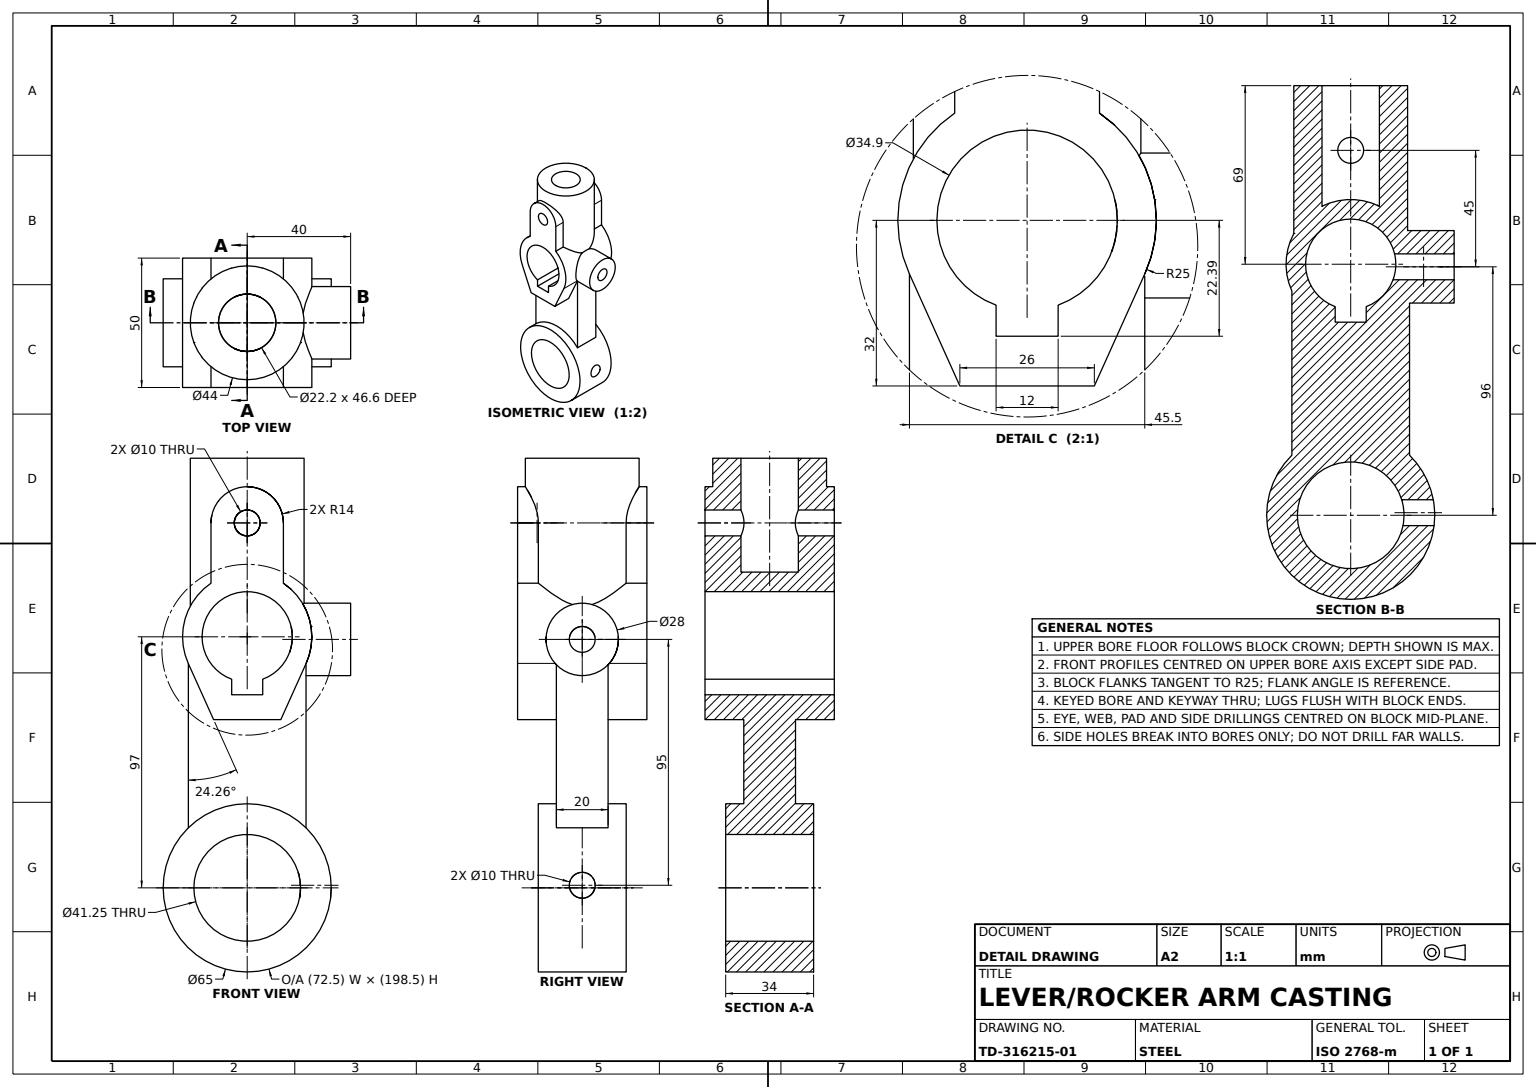
from build123d import *

# Parameters (mm, degrees)
CENTER_BLOCK_DEPTH             = 25
LOWER_EYE_PROFILE_65_R         = 32.5
LOWER_EYE_BOSS_65_DEPTH        = 17
CONNECTING_ARM_PROFILE_W       = 20
CONNECTING_ARM_PROFILE_H       = 65
CONNECTING_ARM_DEPTH           = 22.75
UPPER_BOSS_44_REACH            = 204.691
UPPER_BOSS_44_END_RADIUS       = 25
UPPER_BOSS_PROFILE_44_R        = 22
SIDE_PAD_REACH                 = 144.571
SIDE_PAD_END_RADIUS            = 22
SIDE_PAD_EXTENSION_REACH       = 144.571
UPPER_BORE_22_2_REACH          = 204.691
UPPER_BORE_22_2_END_RADIUS     = 25
UPPER_BORE_PROFILE_22_2_R      = 11.1
LUG_PLATE_REACH                = 152.504
LUG_PLATE_PROFILE_R            = 14
KEYED_SIDE_BORE_PROFILE_R      = 5
KEYED_SIDE_BORE_DEPTH          = 145.465393842
LUG_PIN_HOLE_PROFILE_10_R      = 5
LUG_PIN_HOLE_10_DEPTH          = 45
LOWER_EYE_BORE_PROFILE_41_25_R = 20.625
LOWER_EYE_BORE_41_25_DEPTH     = 45
CROSS_PIN_HOLE_PROFILE_10_R    = 5
CROSS_PIN_HOLE_10_DEPTH        = 100


with BuildPart() as part:
    # Center Block Profile → Center Block (new, symmetric)
    with BuildSketch(Plane.XY):
        with BuildLine():
            Line((-13, -32), (13, -32))
            Line((13, -32), (22.792288735, -10.271882702))
            ThreePointArc((22.792288735, -10.271882702), (0, 25), (-22.792288735, -10.271882702))
            Line((-22.792288735, -10.271882702), (-13, -32))
        make_face()
    extrude(amount=CENTER_BLOCK_DEPTH, both=True)



with BuildPart() as body_2:
    # Lower Eye Profile Ø65 → Lower Eye Boss Ø65 (new, symmetric)
    with BuildSketch(Plane.XY):
        with Locations((0, -97)):
            Circle(LOWER_EYE_PROFILE_65_R)
    extrude(amount=LOWER_EYE_BOSS_65_DEPTH, both=True)


with BuildPart() as part_1:
    add(part.part)

    add(body_2.part)  # Connecting Arm merges body 2
    # Connecting Arm Profile → Connecting Arm (add, symmetric)
    with BuildSketch(Plane(origin=(0, 0, 0), x_dir=(0, 0, -1), z_dir=(1, 0, 0))):
        with Locations((0, -42.771882702)):
            Rectangle(CONNECTING_ARM_PROFILE_W, CONNECTING_ARM_PROFILE_H)
    extrude(amount=CONNECTING_ARM_DEPTH, both=True)

    # Upper Boss Ø44: up to this cylinder (the profile starts outside it)
    upper_boss_44_end = Plane(origin=(0, 0, 0), z_dir=(0, 0, -1)) * Cylinder(UPPER_BOSS_44_END_RADIUS, 460.382, mode=Mode.PRIVATE)
    # Upper Boss Profile Ø44 → Upper Boss Ø44 (add, up to the surface)
    with BuildSketch(Plane(origin=(0, 69, 0), x_dir=(1, 0, 0), z_dir=(0, 1, 0)), mode=Mode.PRIVATE) as upper_boss_44_sk1:
        with Locations(Location((0, 0, 0), (0, 0, 270))):
            Circle(UPPER_BOSS_PROFILE_44_R)
    upper_boss_44_tool1 = extrude(upper_boss_44_sk1.sketch, amount=-UPPER_BOSS_44_REACH, mode=Mode.PRIVATE) - upper_boss_44_end
    add(upper_boss_44_tool1.solids().sort_by_distance((0, 69, 0))[0])

    # Side Pad: up to this cylinder (the profile starts outside it)
    side_pad_end = Plane(origin=(0, 39.439951, 0), z_dir=(0, 1, 0)) * Cylinder(SIDE_PAD_END_RADIUS, 334.142, mode=Mode.PRIVATE)
    # Side Pad Profile → Side Pad (add, up to the surface)
    with BuildSketch(Plane.XY.offset(25), mode=Mode.PRIVATE) as side_pad_sk1:
        with BuildLine():
            Line((-14, 44), (-14, 20.712315177))
            ThreePointArc((-14, 20.712315177), (0, 25), (14, 20.712315177))
            Line((14, 20.712315177), (14, 44))
            ThreePointArc((14, 44), (0, 58), (-14, 44))
        make_face()
    side_pad_tool1 = extrude(side_pad_sk1.sketch, amount=-SIDE_PAD_REACH, mode=Mode.PRIVATE) - side_pad_end
    add(side_pad_tool1.solids().sort_by_distance((0, 39.439951, 25))[0])

    # Side Pad Extension Profile → Side Pad Extension (add, up to next)
    with BuildSketch(Plane(origin=(0, 0, -25), x_dir=(-1, 0, 0), z_dir=(0, 0, -1)), mode=Mode.PRIVATE) as side_pad_extension_sk1:
        with BuildLine():
            Line((-14, 44), (-14, 20.712315177))
            ThreePointArc((-14, 20.712315177), (0, 25), (14, 20.712315177))
            Line((14, 20.712315177), (14, 44))
            ThreePointArc((14, 44), (0, 58), (-14, 44))
        make_face()
    side_pad_extension_tool1 = extrude(side_pad_extension_sk1.sketch, amount=-SIDE_PAD_EXTENSION_REACH, mode=Mode.PRIVATE) - part_1.part
    add(side_pad_extension_tool1.solids().sort_by_distance((0, 39.439951, -25))[0])

    # Upper Bore Ø22.2: up to this cylinder (the profile starts outside it)
    upper_bore_22_2_end = Plane(origin=(0, 0, 0), z_dir=(0, 0, -1)) * Cylinder(UPPER_BORE_22_2_END_RADIUS, 460.382, mode=Mode.PRIVATE)
    # Upper Bore Profile Ø22.2 → Upper Bore Ø22.2 (cut, up to the surface)
    with BuildSketch(Plane(origin=(0, 69, 0), x_dir=(1, 0, 0), z_dir=(0, 1, 0)), mode=Mode.PRIVATE) as upper_bore_22_2_sk1:
        with Locations(Location((0, 0, 0), (0, 0, 270))):
            Circle(UPPER_BORE_PROFILE_22_2_R)
    upper_bore_22_2_tool1 = extrude(upper_bore_22_2_sk1.sketch, amount=-UPPER_BORE_22_2_REACH, mode=Mode.PRIVATE) - upper_bore_22_2_end
    add(upper_bore_22_2_tool1.solids().sort_by_distance((0, 69, 0))[0], mode=Mode.SUBTRACT)

    # Lug Plate Profile → Lug Plate (add, up to next)
    with BuildSketch(Plane(origin=(-40, 0, 0), x_dir=(0, 0, -1), z_dir=(1, 0, 0)), mode=Mode.PRIVATE) as lug_plate_sk1:
        with Locations(Location((0, -1, 0), (0, 0, 221.473787501))):
            Circle(LUG_PLATE_PROFILE_R)
    lug_plate_tool1 = extrude(lug_plate_sk1.sketch, amount=LUG_PLATE_REACH, mode=Mode.PRIVATE) - part_1.part
    add(lug_plate_tool1.solids().sort_by_distance((-40, -1, 0))[0])

    # Keyed Side Bore Profile → Keyed Side Bore (cut, through all)
    with BuildSketch(Plane(origin=(0, 0, -25), x_dir=(-1, 0, 0), z_dir=(0, 0, -1))):
        with Locations((0, 44)):
            Circle(KEYED_SIDE_BORE_PROFILE_R)
        with BuildLine():
            Line((-6, -16.386045893), (-6, -22.39))
            Line((-6, -22.39), (6, -22.39))
            Line((6, -22.39), (6, -16.386045893))
            ThreePointArc((6, -16.386045893), (0, 17.45), (-6, -16.386045893))
        make_face()
    extrude(amount=-KEYED_SIDE_BORE_DEPTH, mode=Mode.SUBTRACT)

    # Lug Pin Hole Profile Ø10 → Lug Pin Hole Ø10 (cut)
    with BuildSketch(Plane.ZY.offset(40)):
        with Locations((0, -1)):
            Circle(LUG_PIN_HOLE_PROFILE_10_R)
    extrude(amount=-LUG_PIN_HOLE_10_DEPTH, mode=Mode.SUBTRACT)

    # Lower Eye Bore Profile Ø41.25 → Lower Eye Bore Ø41.25 (cut)
    with BuildSketch(Plane(origin=(0, 0, -17), x_dir=(-1, 0, 0), z_dir=(0, 0, -1))):
        with Locations((0, -97)):
            Circle(LOWER_EYE_BORE_PROFILE_41_25_R)
    extrude(amount=-LOWER_EYE_BORE_41_25_DEPTH, mode=Mode.SUBTRACT)

    # Cross Pin Hole Profile Ø10 → Cross Pin Hole Ø10 (cut)
    with BuildSketch(Plane(origin=(0, 0, 0), x_dir=(0, 0, -1), z_dir=(1, 0, 0))):
        with Locations(Location((0, -96, 0), (0, 0, 191.536959033))):
            Circle(CROSS_PIN_HOLE_PROFILE_10_R)
    extrude(amount=-CROSS_PIN_HOLE_10_DEPTH, mode=Mode.SUBTRACT)


solid = part_1.part
